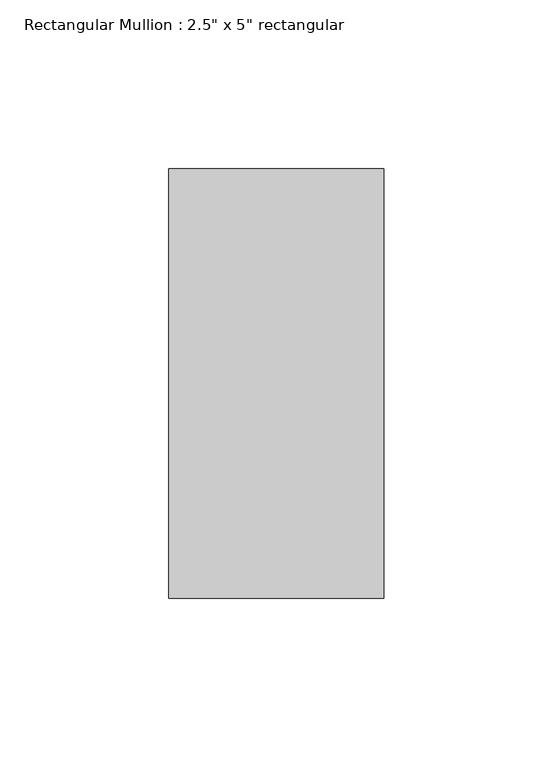
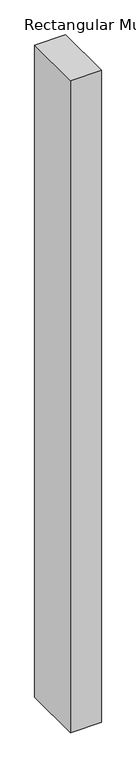
"""IFC4 building model written with IfcOpenShell, lengths in millimetres: member geometry."""

from ifc_helpers import new_model, si_unit, frame, origin, place, context, project, spatial, polyline, outline, extrude, source, transform, mapped, element, save


def member_4b717c4e(model_context):
    return source(origin(), model_context, "Body", "SweptSolid", [
        extrude(outline(polyline([(0.0, 63.5), (0.0, -63.5), (-63.5, -63.5), (-63.5, 63.5), (0.0, 63.5)])), frame((0.0, 0.0, -1416.05), z_axis=(0.0, 0.0, 1.0), x_axis=(1.0, 0.0, 0.0)), (0.0, 0.0, 1.0), 1416.05),
    ])


if __name__ == "__main__":
    model = new_model("IFC4")
    model_context = context("Model", 3, world=origin())
    ifc_project = project(units=[si_unit("LENGTHUNIT", "METRE", prefix="MILLI")], contexts=[model_context])
    site = spatial("IfcSite", under=ifc_project)
    building = spatial("IfcBuilding", under=site)
    placement = place(None, origin())
    member_shape = member_4b717c4e(model_context)
    element("IfcMember", 1, ObjectType="Rectangular Mullion : 2.5\" x 5\" rectangular", at=placement, inside=building, context=model_context, shape_type="MappedRepresentation", body=[
        mapped(member_shape, transform((0.0, 0.0, 0.0), x_axis=(1.0, 0.0, 0.0), y_axis=(0.0, 1.0, 0.0), z_axis=(0.0, 0.0, 1.0))),
    ])
    save(model, "model.ifc")

# Revit data of these elements
# Type "Rectangular Mullion : 2.5\" x 5\" rectangular"
#   built-in parameter 1007304 = 0.416667 (stored number, unit not read)
#   built-in parameter 1007301 = 0.104167 (stored number, unit not read)
#   built-in parameter 1007300 = 0.104167 (stored number, unit not read)
# Element 1 (IfcMember, "Rectangular Mullion : 2.5\" x 5\" rectangular")
#   Materials on its faces: "Aluminum"
# Materials
#   "Aluminum": class "Metal", colour RGB 247 247 247, transparency 0, Description = "Aluminum 6061", Cost = 0
